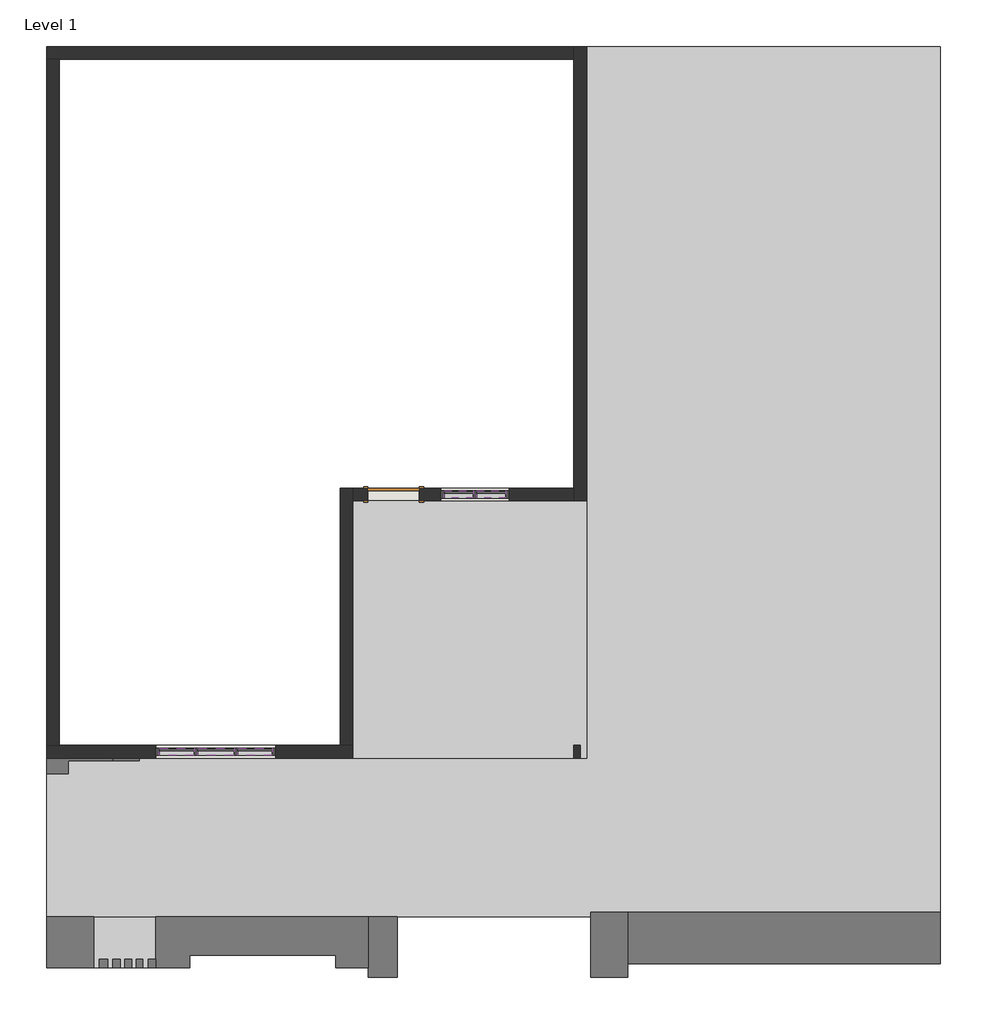
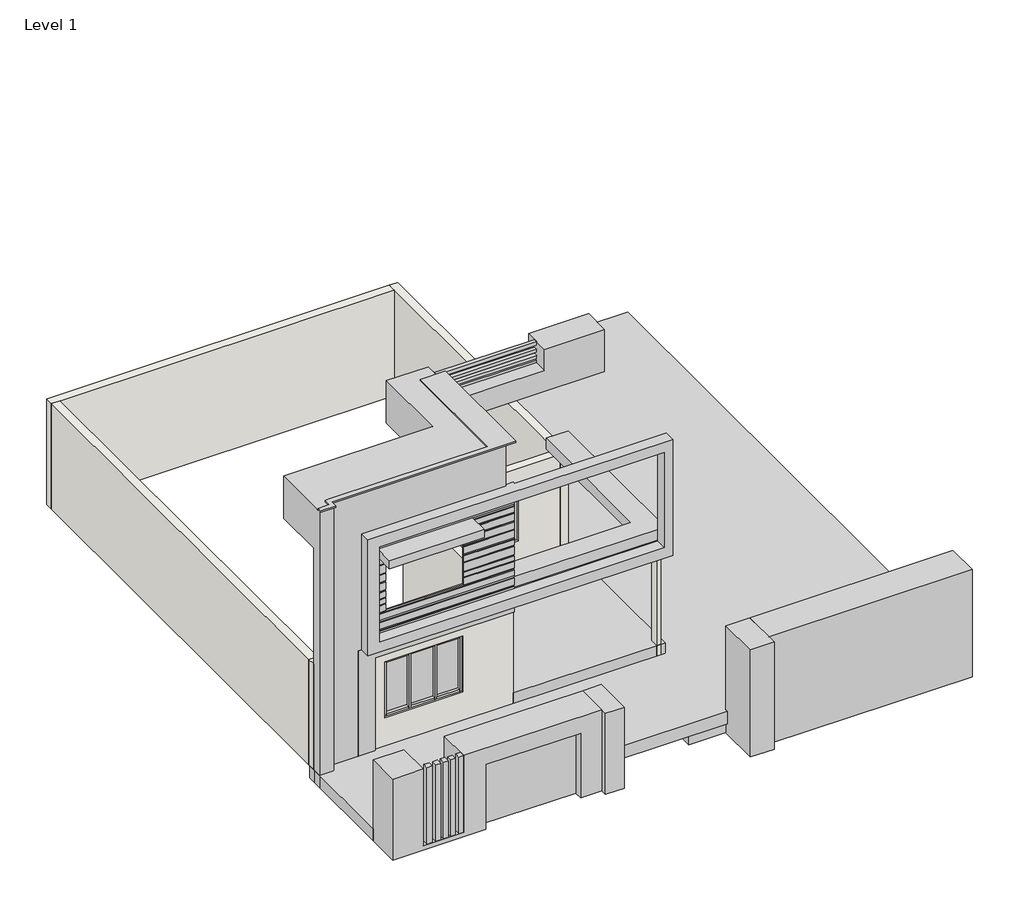
# One storey: 17 members, 7 walls, 5 plates, 1 door, 1 proxy.
"""IFC4 building model written with IfcOpenShell, lengths in millimetres."""

from ifc_helpers import new_model, si_unit, frame, origin, origin_with_axes, place, context, project, spatial, polyline, outline, extrude, faceted_brep, transform, mapped, element, save
from components import generic_models_1_generic_models_1_c55d1f28, door_0ca8825f, member_3f0e0172, member_5215b92c, member_74b724cb, member_40397874, member_0b7646a3, member_4c43c051, member_e1556d54, system_panel_glazed_6ea480bf, system_panel_glazed_43ab5a70, system_panel_glazed_e08f8b61

model = new_model("IFC4")

# Units and contexts
model_context = context("Model", 3, world=origin())
ifc_project = project(units=[si_unit("LENGTHUNIT", "METRE", prefix="MILLI")], contexts=[model_context])

# Site, building, storey
site = spatial("IfcSite", under=ifc_project)
building = spatial("IfcBuilding", under=site)
storey = spatial("IfcBuildingStorey", under=building, Name="Level 1", Elevation=0.0)

# Proxy
placement = place(None, origin())
generic_models_1_generic_models_1_shape = generic_models_1_generic_models_1_c55d1f28(model_context)
element("IfcBuildingElementProxy", 1, Name="Generic Models 1 : Generic Models 1", ObjectType="Generic Models 1 : Generic Models 1", at=placement, inside=storey, context=model_context, shape_type="MappedRepresentation", body=[
    mapped(generic_models_1_generic_models_1_shape, transform((0.0, 0.0, 0.0), x_axis=(1.0, 0.0, 0.0), y_axis=(0.0, 1.0, 0.0), z_axis=(0.0, 0.0, 1.0))),
])

# Door
door_shape = door_0ca8825f(model_context)
element("IfcDoor", 2, ObjectType="Single-Flush : 36\" x 84\"", at=placement, inside=storey, context=model_context, shape_type="MappedRepresentation", body=[
    mapped(door_shape, transform((-11006.187855, -7781.0768247, 152.4), x_axis=(1.0, 0.0, 0.0), y_axis=(0.0, 1.0, 0.0), z_axis=(0.0, 0.0, 1.0))),
])

# Members
member_shape = member_3f0e0172(model_context)
element("IfcMember", 3, ObjectType="Rectangular Mullion : 2.5\" x 5\" rectangular", at=placement, inside=storey, context=model_context, shape_type="MappedRepresentation", body=[
    mapped(member_shape, transform((-13781.137855, -12353.0768247, 816.4614273), x_axis=(0.0, 0.0, -1.0), y_axis=(0.0, -1.0, 0.0), z_axis=(-1.0, 0.0, 0.0))),
])
element("IfcMember", 4, ObjectType="Rectangular Mullion : 2.5\" x 5\" rectangular", at=placement, inside=storey, context=model_context, shape_type="MappedRepresentation", body=[
    mapped(member_shape, transform((-15171.787855, -12353.0768247, 816.4614273), x_axis=(0.0, 0.0, -1.0), y_axis=(0.0, -1.0, 0.0), z_axis=(-1.0, 0.0, 0.0))),
])
member_2_shape = member_5215b92c(model_context)
element("IfcMember", 5, ObjectType="Rectangular Mullion : 2.5\" x 5\" rectangular", at=placement, inside=storey, context=model_context, shape_type="MappedRepresentation", body=[
    mapped(member_2_shape, transform((-14492.337855, -12353.0768247, 816.4614273), x_axis=(0.0, 0.0, -1.0), y_axis=(0.0, -1.0, 0.0), z_axis=(-1.0, 0.0, 0.0))),
])
member_3_shape = member_74b724cb(model_context)
element("IfcMember", 6, ObjectType="Rectangular Mullion : 2.5\" x 5\" rectangular", at=placement, inside=storey, context=model_context, shape_type="MappedRepresentation", body=[
    mapped(member_3_shape, transform((-14524.087855, -12353.0768247, 816.4614273), x_axis=(1.0, 0.0, 0.0), y_axis=(0.0, -1.0, 0.0), z_axis=(0.0, 0.0, -1.0))),
])
element("IfcMember", 7, ObjectType="Rectangular Mullion : 2.5\" x 5\" rectangular", at=placement, inside=storey, context=model_context, shape_type="MappedRepresentation", body=[
    mapped(member_3_shape, transform((-13812.887855, -12353.0768247, 816.4614273), x_axis=(1.0, 0.0, 0.0), y_axis=(0.0, -1.0, 0.0), z_axis=(0.0, 0.0, -1.0))),
])
element("IfcMember", 8, ObjectType="Rectangular Mullion : 2.5\" x 5\" rectangular", at=placement, inside=storey, context=model_context, shape_type="MappedRepresentation", body=[
    mapped(member_2_shape, transform((-13844.637855, -12353.0768247, 2433.8714904), x_axis=(0.0, 0.0, 1.0), y_axis=(0.0, -1.0, 0.0), z_axis=(1.0, 0.0, 0.0))),
])
element("IfcMember", 9, ObjectType="Rectangular Mullion : 2.5\" x 5\" rectangular", at=placement, inside=storey, context=model_context, shape_type="MappedRepresentation", body=[
    mapped(member_shape, transform((-14555.837855, -12353.0768247, 2433.8714904), x_axis=(0.0, 0.0, 1.0), y_axis=(0.0, -1.0, 0.0), z_axis=(1.0, 0.0, 0.0))),
])
element("IfcMember", 10, ObjectType="Rectangular Mullion : 2.5\" x 5\" rectangular", at=placement, inside=storey, context=model_context, shape_type="MappedRepresentation", body=[
    mapped(member_shape, transform((-13165.187855, -12353.0768247, 2433.8714904), x_axis=(0.0, 0.0, 1.0), y_axis=(0.0, -1.0, 0.0), z_axis=(1.0, 0.0, 0.0))),
])
member_4_shape = member_40397874(model_context)
element("IfcMember", 11, ObjectType="Rectangular Mullion : 2.5\" x 5\" rectangular", at=placement, inside=storey, context=model_context, shape_type="MappedRepresentation", body=[
    mapped(member_4_shape, transform((-15235.287855, -12353.0768247, 2433.8714904), x_axis=(-1.0, 0.0, 0.0), y_axis=(0.0, -1.0, 0.0), z_axis=(0.0, 0.0, 1.0))),
])
element("IfcMember", 12, ObjectType="Rectangular Mullion : 2.5\" x 5\" rectangular", at=placement, inside=storey, context=model_context, shape_type="MappedRepresentation", body=[
    mapped(member_4_shape, transform((-13101.687855, -12353.0768247, 816.4614273), x_axis=(1.0, 0.0, 0.0), y_axis=(0.0, -1.0, 0.0), z_axis=(0.0, 0.0, -1.0))),
])
member_5_shape = member_0b7646a3(model_context)
element("IfcMember", 13, ObjectType="Rectangular Mullion : 2.5\" x 5\" rectangular", at=placement, inside=storey, context=model_context, shape_type="MappedRepresentation", body=[
    mapped(member_5_shape, transform((-9526.637855, -7781.0768247, 960.4474363), x_axis=(0.0, 0.0, -1.0), y_axis=(0.0, -1.0, 0.0), z_axis=(-1.0, 0.0, 0.0))),
])
element("IfcMember", 14, ObjectType="Rectangular Mullion : 2.5\" x 5\" rectangular", at=placement, inside=storey, context=model_context, shape_type="MappedRepresentation", body=[
    mapped(member_5_shape, transform((-10104.487855, -7781.0768247, 960.4474363), x_axis=(0.0, 0.0, -1.0), y_axis=(0.0, -1.0, 0.0), z_axis=(-1.0, 0.0, 0.0))),
])
member_6_shape = member_4c43c051(model_context)
element("IfcMember", 15, ObjectType="Rectangular Mullion : 2.5\" x 5\" rectangular", at=placement, inside=storey, context=model_context, shape_type="MappedRepresentation", body=[
    mapped(member_6_shape, transform((-9558.387855, -7781.0768247, 960.4474363), x_axis=(1.0, 0.0, 0.0), y_axis=(0.0, -1.0, 0.0), z_axis=(0.0, 0.0, -1.0))),
])
element("IfcMember", 16, ObjectType="Rectangular Mullion : 2.5\" x 5\" rectangular", at=placement, inside=storey, context=model_context, shape_type="MappedRepresentation", body=[
    mapped(member_5_shape, transform((-9590.137855, -7781.0768247, 2370.8419829), x_axis=(0.0, 0.0, 1.0), y_axis=(0.0, -1.0, 0.0), z_axis=(1.0, 0.0, 0.0))),
])
element("IfcMember", 17, ObjectType="Rectangular Mullion : 2.5\" x 5\" rectangular", at=placement, inside=storey, context=model_context, shape_type="MappedRepresentation", body=[
    mapped(member_5_shape, transform((-9012.287855, -7781.0768247, 2370.8419829), x_axis=(0.0, 0.0, 1.0), y_axis=(0.0, -1.0, 0.0), z_axis=(1.0, 0.0, 0.0))),
])
member_7_shape = member_e1556d54(model_context)
element("IfcMember", 18, ObjectType="Rectangular Mullion : 2.5\" x 5\" rectangular", at=placement, inside=storey, context=model_context, shape_type="MappedRepresentation", body=[
    mapped(member_7_shape, transform((-10167.987855, -7781.0768247, 2370.8419829), x_axis=(-1.0, 0.0, 0.0), y_axis=(0.0, -1.0, 0.0), z_axis=(0.0, 0.0, 1.0))),
])
element("IfcMember", 19, ObjectType="Rectangular Mullion : 2.5\" x 5\" rectangular", at=placement, inside=storey, context=model_context, shape_type="MappedRepresentation", body=[
    mapped(member_7_shape, transform((-8948.787855, -7781.0768247, 960.4474363), x_axis=(1.0, 0.0, 0.0), y_axis=(0.0, -1.0, 0.0), z_axis=(0.0, 0.0, -1.0))),
])

# Plates
system_panel_glazed_shape = system_panel_glazed_6ea480bf(model_context)
element("IfcPlate", 20, ObjectType="System Panel : Glazed", at=placement, inside=storey, context=model_context, shape_type="MappedRepresentation", body=[
    mapped(system_panel_glazed_shape, transform((-14863.812855, -12353.0768247, 879.9614273), x_axis=(1.0, 0.0, 0.0), y_axis=(0.0, 1.0, 0.0), z_axis=(0.0, 0.0, 1.0))),
])
element("IfcPlate", 21, ObjectType="System Panel : Glazed", at=placement, inside=storey, context=model_context, shape_type="MappedRepresentation", body=[
    mapped(system_panel_glazed_shape, transform((-13473.162855, -12353.0768247, 879.9614273), x_axis=(1.0, 0.0, 0.0), y_axis=(0.0, 1.0, 0.0), z_axis=(0.0, 0.0, 1.0))),
])
system_panel_glazed_2_shape = system_panel_glazed_43ab5a70(model_context)
element("IfcPlate", 22, ObjectType="System Panel : Glazed", at=placement, inside=storey, context=model_context, shape_type="MappedRepresentation", body=[
    mapped(system_panel_glazed_2_shape, transform((-14168.487855, -12353.0768247, 879.9614273), x_axis=(1.0, 0.0, 0.0), y_axis=(0.0, 1.0, 0.0), z_axis=(0.0, 0.0, 1.0))),
])
system_panel_glazed_3_shape = system_panel_glazed_e08f8b61(model_context)
element("IfcPlate", 23, ObjectType="System Panel : Glazed", at=placement, inside=storey, context=model_context, shape_type="MappedRepresentation", body=[
    mapped(system_panel_glazed_3_shape, transform((-9847.312855, -7781.0768247, 1023.9474363), x_axis=(1.0, 0.0, 0.0), y_axis=(0.0, 1.0, 0.0), z_axis=(0.0, 0.0, 1.0))),
])
element("IfcPlate", 24, ObjectType="System Panel : Glazed", at=placement, inside=storey, context=model_context, shape_type="MappedRepresentation", body=[
    mapped(system_panel_glazed_3_shape, transform((-9269.462855, -7781.0768247, 1023.9474363), x_axis=(1.0, 0.0, 0.0), y_axis=(0.0, 1.0, 0.0), z_axis=(0.0, 0.0, 1.0))),
])

# Walls
element("IfcWall", 25, ObjectType="9\"", at=placement, inside=storey, context=model_context, shape_type="Brep", body=[
    faceted_brep([(-17178.387855, -12467.3768247, 0.0), (-11730.087855, -12467.3768247, 0.0), (-11730.087855, -12467.3768247, 3048.0), (-17178.387855, -12467.3768247, 3048.0), (-15235.287855, -12467.3768247, 816.4614273), (-15235.287855, -12467.3768247, 2433.8714904), (-13101.687855, -12467.3768247, 2433.8714904), (-13101.687855, -12467.3768247, 816.4614273), (-11730.087855, -12238.7768247, 0.0), (-11958.687855, -12238.7768247, 0.0), (-16949.787855, -12238.7768247, 0.0), (-17178.387855, -12238.7768247, 0.0), (-17178.387855, -12238.7768247, 3048.0), (-16949.787855, -12238.7768247, 3048.0), (-11958.687855, -12238.7768247, 3048.0), (-11730.087855, -12238.7768247, 3048.0), (-15235.287855, -12238.7768247, 2433.8714904), (-15235.287855, -12238.7768247, 816.4614273), (-13101.687855, -12238.7768247, 816.4614273), (-13101.687855, -12238.7768247, 2433.8714904)], [[[0, 1, 2, 3], [4, 5, 6, 7]], [[8, 9, 10, 11, 12, 13, 14, 15], [16, 17, 18, 19]], [[1, 0, 11, 10, 9, 8]], [[2, 1, 8, 15]], [[3, 2, 15, 14, 13, 12]], [[0, 3, 12, 11]], [[4, 17, 16, 5]], [[5, 16, 19, 6]], [[6, 19, 18, 7]], [[17, 4, 7, 18]]]),
])
element("IfcWall", 26, ObjectType="9\"", at=placement, inside=storey, context=model_context, shape_type="Brep", body=[
    faceted_brep([(-7805.787855, 181.8231753, 0.0), (-17178.387855, 181.8231753, 0.0), (-17178.387855, 181.8231753, 3048.0), (-7805.787855, 181.8231753, 3048.0), (-7805.787855, -46.7768247, 0.0), (-7805.787855, -46.7768247, 3048.0), (-16949.787855, -46.7768247, 3048.0), (-17178.387855, -46.7768247, 3048.0), (-17178.387855, -46.7768247, 0.0), (-16949.787855, -46.7768247, 0.0)], [[[0, 1, 2, 3]], [[4, 5, 6, 7, 8, 9]], [[1, 0, 4, 9, 8]], [[3, 2, 7, 6, 5]], [[0, 3, 5, 4]], [[2, 1, 8, 7]]]),
])
element("IfcWall", 27, ObjectType="9\"", at=placement, inside=storey, context=model_context, shape_type="SweptSolid", body=[
    extrude(outline(polyline([(-17178.387855, -12238.7768247), (-17178.387855, -46.7768247), (-16949.787855, -46.7768247), (-16949.787855, -12238.7768247), (-17178.387855, -12238.7768247)])), origin_with_axes(), (0.0, 0.0, 1.0), 3048.0),
])
element("IfcWall", 28, ObjectType="9\"", at=placement, inside=storey, context=model_context, shape_type="Brep", body=[
    faceted_brep([(-11730.087855, -12238.7768247, 0.0), (-11730.087855, -7895.3768247, 0.0), (-11730.087855, -7666.7768247, 0.0), (-11730.087855, -7666.7768247, 3048.0), (-11730.087855, -7895.3768247, 3048.0), (-11730.087855, -12238.7768247, 3048.0), (-11958.687855, -12238.7768247, 0.0), (-11958.687855, -12238.7768247, 3048.0), (-11958.687855, -7666.7768247, 3048.0), (-11958.687855, -7666.7768247, 0.0)], [[[0, 1, 2, 3, 4, 5]], [[6, 7, 8, 9]], [[2, 1, 0, 6, 9]], [[5, 4, 3, 8, 7]], [[0, 5, 7, 6]], [[3, 2, 9, 8]]]),
])
element("IfcWall", 29, ObjectType="9\"", at=placement, inside=storey, context=model_context, shape_type="SweptSolid", body=[
    extrude(outline(polyline([(0.0, -11730.087855), (0.0, -7805.787855), (3048.0, -7805.787855), (3048.0, -11730.087855), (0.0, -11730.087855)]), holes=[polyline([(960.4474363, -10167.987855), (2370.8419829, -10167.987855), (2370.8419829, -8948.787855), (960.4474363, -8948.787855), (960.4474363, -10167.987855)]), polyline([(152.4, -10548.987855), (152.4, -11463.387855), (2286.0, -11463.387855), (2286.0, -10548.987855), (152.4, -10548.987855)])]), frame((0.0, -7895.3768247, 0.0), z_axis=(0.0, 1.0, 0.0), x_axis=(0.0, 0.0, 1.0)), (0.0, 0.0, 1.0), 228.6),
])
element("IfcWall", 30, ObjectType="9\"", at=placement, inside=storey, context=model_context, shape_type="SweptSolid", body=[
    extrude(outline(polyline([(-7691.487855, -12467.3768247), (-7805.787855, -12467.3768247), (-7805.787855, -12238.7768247), (-7691.487855, -12238.7768247), (-7691.487855, -12467.3768247)])), origin_with_axes(), (0.0, 0.0, 1.0), 3048.0),
])
element("IfcWall", 31, ObjectType="9\"", at=placement, inside=storey, context=model_context, shape_type="Brep", body=[
    faceted_brep([(-7577.187855, -7895.3768247, 0.0), (-7577.187855, 181.8231753, 0.0), (-7577.187855, 181.8231753, 3048.0), (-7577.187855, -7895.3768247, 3048.0), (-7805.787855, -7895.3768247, 0.0), (-7805.787855, -7895.3768247, 3048.0), (-7805.787855, -7666.7768247, 3048.0), (-7805.787855, -46.7768247, 3048.0), (-7805.787855, 181.8231753, 3048.0), (-7805.787855, 181.8231753, 0.0), (-7805.787855, -46.7768247, 0.0), (-7805.787855, -7666.7768247, 0.0)], [[[0, 1, 2, 3]], [[4, 5, 6, 7, 8, 9, 10, 11]], [[1, 0, 4, 11, 10, 9]], [[3, 2, 8, 7, 6, 5]], [[0, 3, 5, 4]], [[2, 1, 9, 8]]]),
])

save(model, "model.ifc")

# Revit data of these elements
# Type "Single-Flush : 36\" x 84\""
#   Type Mark = "1"
#   Construction Type Id = "MDOOR"
#   Assembly Code = "C1020"
#   Analytic Construction = "Metal"
#   Thickness = 0' - 2"
#   Heat Transfer Coefficient (U) = 0.651978 BTU/(h·ft²·°F)
#   Height = 7' - 0"
#   Trim Projection Ext = 0' - 1"
#   Trim Projection Int = 0' - 1"
#   Trim Width = 0' - 3"
#   Width = 3' - 0"
#   Define Thermal Properties by = 1
#   Define Thermal Properties by = 1
#   Door Material = Door - Panel
#   Frame Material = Door - Frame
#   Visual Light Transmittance = 0
#   Solar Heat Gain Coefficient = 0
#   Function = (empty or 0)
#   Wall Closure = (empty or 0)
# Type "Rectangular Mullion : 2.5\" x 5\" rectangular"
#   built-in parameter 1007304 = 0.416667 (stored number, unit not read)
#   built-in parameter 1007301 = 0.104167 (stored number, unit not read)
#   built-in parameter 1007300 = 0.104167 (stored number, unit not read)
# Type "System Panel : Glazed"
#   Construction Type Id = "GSP4R"
#   Analytic Construction = "1/8 in Pilkington single glazing"
#   Visual Light Transmittance = 0.9
#   Solar Heat Gain Coefficient = 0.86
#   Heat Transfer Coefficient (U) = 1.18115 BTU/(h·ft²·°F)
#   Define Thermal Properties by = 1
# Type "9\""
#   Assembly Code = "B2010"
#   Layers, outside or top first: 0' - 9" no material (function 1)
# Element 1 (IfcBuildingElementProxy, "Generic Models 1 : Generic Models 1")
#   Phase Created = New Construction
# Element 2 (IfcDoor, "Single-Flush : 36\" x 84\"")
#   Phase Created = New Construction
#   Materials on its faces: "Door - Frame", "Door - Panel"
# Elements 3, 4, 5, 6, 7, 8, 9, 10, 11, 12, 13, 14, 15, 16, 17, 18, 19 (IfcMember, "Rectangular Mullion : 2.5\" x 5\" rectangular")
#   Phase Created = New Construction
#   Materials on its faces: "Aluminum"
# Elements 20, 21, 22, 23, 24 (IfcPlate, "System Panel : Glazed")
#   Phase Created = New Construction
#   Materials on its faces: "Glass"
# Elements 25, 26, 27, 28, 29, 30, 31 (IfcWall, "9\"")
#   Top Offset = 0' - 0"
#   Base Offset = 0' - 0"
#   Unconnected Height = 10' - 0"
#   wall height = 10' - 0"
#   Phase Created = New Construction
#   Base Constraint = Level 1
#   Materials on its faces: "Default Wall"
# Materials
#   "Door - Panel": class "Wood", colour RGB 210 159 95, transparency 0, Cost = 0
#   "Door - Frame": colour RGB 118 70 51, transparency 0, Cost = 0
#   "Aluminum": class "Metal", colour RGB 247 247 247, transparency 0, Description = "Aluminum 6061", Cost = 0
#   "Glass": class "Glass", colour RGB 0 128 192, transparency 0.75, Description = "Soda Lime Glass", Cost = 0
#   "Default Wall": colour RGB 128 128 128, transparency 0, Cost = 0
